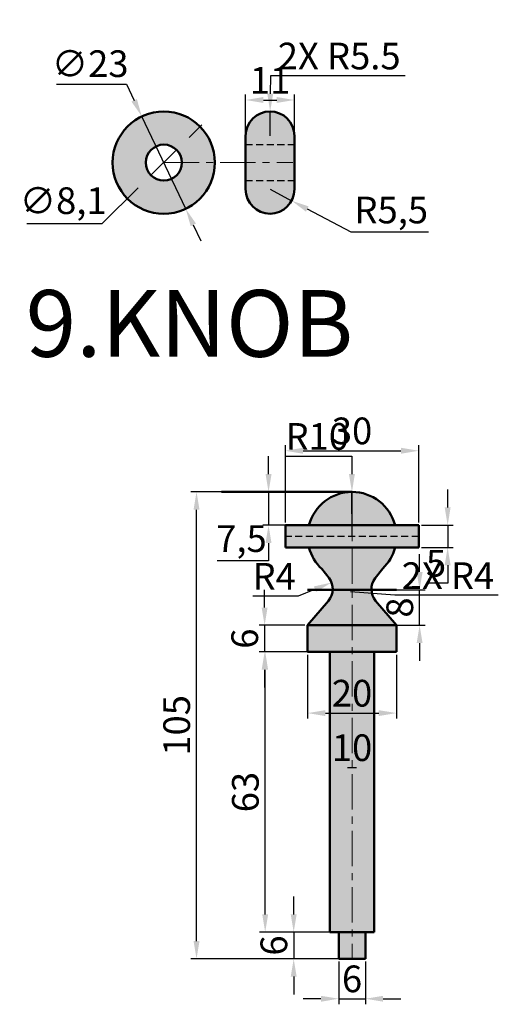
# Model space of a CAD drawing. Units: millimetres. Extents: x -14 to 1073, y -445 to 318.
# Tile 5 of 6: x 615 to 723, y -42 to 179. Entities that reach past the tile are written whole.
import ezdxf

# ---------------------------------------------------------------- set-up
doc = ezdxf.new("R2010")
doc.units = ezdxf.units.MM
doc.header["$LTSCALE"] = 0.5
doc.linetypes.add('CENTER', pattern=[50.8, 31.75, -6.35, 6.35, -6.35])
doc.linetypes.add('HIDDEN', pattern=[9.525, 6.35, -3.175])
for name, color, linetype, lineweight in [('M-CNTR', 1, 'CENTER', 18), ('M-DIMS', 2, 'Continuous', 25), ('M-HATC', 8, 'Continuous', 18), ('M-HIDN', 4, 'HIDDEN', 25), ('M-OUTL', 7, 'Continuous', 50), ('M-TEXT', 3, 'Continuous', 25)]:
    doc.layers.add(name, color=color, linetype=linetype, lineweight=lineweight)
doc.styles.get("Standard").update_dxf_attribs({"font": 'arial.ttf'})
doc.dimstyles.new('ISO-25', dxfattribs={"dimtxt": 6, "dimasz": 4, "dimexe": 1.25, "dimexo": 0.625, "dimtad": 1, "dimtoh": 1, "dimtxsty": 'Standard', "dimcen": 2.5, "dimadec": 0, "dimazin": 0, "dimtfac": 1, "dimtmove": 0, "dimatfit": 3, "dimfxl": 1, "dimarcsym": 0})

# ---------------------------------------------------------------- blocks, each defined once
blk = doc.blocks.new('*D47')
at = {"layer": 'Defpoints', "color": 0, "ltscale": 0.5, "transparency": 16777216}
for p in [(642.43, 157.61), (652.3, 136.84)]:
    blk.add_point(p, dxfattribs=at)
at = {"layer": 'M-DIMS', "color": 0, "lineweight": -2, "ltscale": 0.5, "transparency": 16777216}
for p, q in [((623.25, 164.84), (639, 164.84)), ((639, 164.84), (640.72, 161.22)), ((652.3, 136.84), (642.43, 157.61)), ((654.02, 133.22), (655.74, 129.61))]:
    blk.add_line(p, q, dxfattribs=at)
at = {"layer": 'M-DIMS', "color": 0, "ltscale": 0.5, "transparency": 16777216}
for points in [[(641.32, 161.51), (640.11, 160.94), (642.43, 157.61)], [(654.62, 133.51), (653.42, 132.94), (652.3, 136.84)]]:
    blk.add_solid(points, dxfattribs=at)
at = {"layer": 'M-DIMS', "color": 0, "ltscale": 0.5, "transparency": 16777216, "insert": (630.81, 168.69), "char_height": 6, "attachment_point": 5}
blk.add_mtext('∅23', dxfattribs=at)
blk = doc.blocks.new('*D48')
at = {"layer": 'Defpoints', "color": 0, "ltscale": 0.5, "transparency": 16777216}
for p in [(671.27, 141.22), (676.13, 138.66)]:
    blk.add_point(p, dxfattribs=at)
at = {"layer": 'M-DIMS', "color": 0, "lineweight": -2, "ltscale": 0.5, "transparency": 16777216}
for p, q in [((671.27, 141.22), (676.13, 138.66)), ((689.56, 131.57), (679.67, 136.79)), ((706.9, 131.57), (689.56, 131.57))]:
    blk.add_line(p, q, dxfattribs=at)
at = {"layer": 'M-DIMS', "color": 0, "ltscale": 0.5, "transparency": 16777216}
blk.add_solid([(679.98, 137.38), (679.36, 136.2), (676.13, 138.66)], dxfattribs=at)
at = {"layer": 'M-DIMS', "color": 0, "ltscale": 0.5, "transparency": 16777216, "insert": (698.54, 135.78), "char_height": 6, "attachment_point": 5}
blk.add_mtext('R5,5', dxfattribs=at)
blk = doc.blocks.new('*D49')
at = {"layer": 'Defpoints', "color": 0, "ltscale": 0.5, "transparency": 16777216}
for p in [(676.77, 161.3), (665.77, 147.22), (676.77, 147.22)]:
    blk.add_point(p, dxfattribs=at)
at = {"layer": 'M-DIMS', "color": 0, "lineweight": -2, "ltscale": 0.5, "transparency": 16777216}
for p, q in [((665.77, 147.85), (665.77, 162.55)), ((676.77, 147.85), (676.77, 162.55)), ((669.77, 161.3), (672.77, 161.3))]:
    blk.add_line(p, q, dxfattribs=at)
at = {"layer": 'M-DIMS', "color": 0, "ltscale": 0.5, "transparency": 16777216}
for points in [[(669.77, 161.97), (669.77, 160.64), (665.77, 161.3)], [(672.77, 161.97), (672.77, 160.64), (676.77, 161.3)]]:
    blk.add_solid(points, dxfattribs=at)
at = {"layer": 'M-DIMS', "color": 0, "ltscale": 0.5, "transparency": 16777216, "insert": (671.27, 164.94), "char_height": 6, "attachment_point": 5}
blk.add_mtext('11', dxfattribs=at)
blk = doc.blocks.new('*D50')
at = {"layer": 'Defpoints', "color": 0, "ltscale": 0.5, "transparency": 16777216}
for p in [(650.25, 150.07), (644.48, 144.38)]:
    blk.add_point(p, dxfattribs=at)
at = {"layer": 'M-DIMS', "color": 0, "lineweight": -2, "ltscale": 0.5, "transparency": 16777216}
for p, q in [((653.1, 152.87), (655.95, 155.68)), ((650.25, 150.07), (644.48, 144.38)), ((633.51, 133.56), (641.63, 141.57)), ((616.59, 133.56), (633.51, 133.56))]:
    blk.add_line(p, q, dxfattribs=at)
at = {"layer": 'M-DIMS', "color": 0, "ltscale": 0.5, "transparency": 16777216}
for points in [[(652.63, 153.35), (653.57, 152.4), (650.25, 150.07)], [(641.17, 142.05), (642.1, 141.1), (644.48, 144.38)]]:
    blk.add_solid(points, dxfattribs=at)
at = {"layer": 'M-DIMS', "color": 0, "ltscale": 0.5, "transparency": 16777216, "insert": (624.74, 137.89), "char_height": 6, "attachment_point": 5}
blk.add_mtext('∅8,1', dxfattribs=at)
blk = doc.blocks.new('*D51')
at = {"layer": 'Defpoints', "color": 0, "ltscale": 0.5, "transparency": 16777216}
for p in [(689.72, -25.82), (676.6, -31.82), (689.72, -31.82)]:
    blk.add_point(p, dxfattribs=at)
at = {"layer": 'M-DIMS', "color": 0, "lineweight": -2, "ltscale": 0.5, "transparency": 16777216}
for p, q in [((676.6, -21.82), (676.6, -17.82)), ((689.1, -25.82), (675.35, -25.82)), ((676.6, -25.82), (676.6, -31.82)), ((689.1, -31.82), (675.35, -31.82)), ((676.6, -35.82), (676.6, -39.82))]:
    blk.add_line(p, q, dxfattribs=at)
at = {"layer": 'M-DIMS', "color": 0, "ltscale": 0.5, "transparency": 16777216}
for points in [[(675.93, -21.82), (677.27, -21.82), (676.6, -25.82)], [(675.93, -35.82), (677.27, -35.82), (676.6, -31.82)]]:
    blk.add_solid(points, dxfattribs=at)
at = {"layer": 'M-DIMS', "color": 0, "ltscale": 0.5, "transparency": 16777216, "insert": (672.91, -28.82), "char_height": 6, "attachment_point": 5, "rotation": 90}
blk.add_mtext('6', dxfattribs=at)
blk = doc.blocks.new('*D52')
at = {"layer": 'Defpoints', "color": 0, "ltscale": 0.5, "transparency": 16777216}
for p in [(654.74, 73.18), (689.72, 73.18), (689.72, -31.82)]:
    blk.add_point(p, dxfattribs=at)
at = {"layer": 'M-DIMS', "color": 0, "lineweight": -2, "ltscale": 0.5, "transparency": 16777216}
for p, q in [((689.1, 73.18), (653.49, 73.18)), ((654.74, -27.82), (654.74, 69.18)), ((689.1, -31.82), (653.49, -31.82))]:
    blk.add_line(p, q, dxfattribs=at)
at = {"layer": 'M-DIMS', "color": 0, "ltscale": 0.5, "transparency": 16777216}
for points in [[(654.07, 69.18), (655.41, 69.18), (654.74, 73.18)], [(654.07, -27.82), (655.41, -27.82), (654.74, -31.82)]]:
    blk.add_solid(points, dxfattribs=at)
at = {"layer": 'M-DIMS', "color": 0, "ltscale": 0.5, "transparency": 16777216, "insert": (651.05, 20.68), "char_height": 6, "attachment_point": 5, "rotation": 90}
blk.add_mtext('105', dxfattribs=at)
blk = doc.blocks.new('*D53')
at = {"layer": 'Defpoints', "color": 0, "ltscale": 0.5, "transparency": 16777216}
for p in [(679.72, 43.18), (670.05, 37.18), (679.72, 37.18)]:
    blk.add_point(p, dxfattribs=at)
at = {"layer": 'M-DIMS', "color": 0, "lineweight": -2, "ltscale": 0.5, "transparency": 16777216}
for p, q in [((670.05, 47.18), (670.05, 51.18)), ((679.1, 43.18), (668.8, 43.18)), ((670.05, 43.18), (670.05, 37.18)), ((679.1, 37.18), (668.8, 37.18)), ((670.05, 33.18), (670.05, 29.18))]:
    blk.add_line(p, q, dxfattribs=at)
at = {"layer": 'M-DIMS', "color": 0, "ltscale": 0.5, "transparency": 16777216}
for points in [[(669.39, 47.18), (670.72, 47.18), (670.05, 43.18)], [(669.39, 33.18), (670.72, 33.18), (670.05, 37.18)]]:
    blk.add_solid(points, dxfattribs=at)
at = {"layer": 'M-DIMS', "color": 0, "ltscale": 0.5, "transparency": 16777216, "insert": (666.36, 40.18), "char_height": 6, "attachment_point": 5, "rotation": 90}
blk.add_mtext('6', dxfattribs=at)
blk = doc.blocks.new('*D54')
at = {"layer": 'Defpoints', "color": 0, "ltscale": 0.5, "transparency": 16777216}
for p in [(670.19, 37.18), (684.72, 37.18), (684.72, -25.82)]:
    blk.add_point(p, dxfattribs=at)
at = {"layer": 'M-DIMS', "color": 0, "lineweight": -2, "ltscale": 0.5, "transparency": 16777216}
for p, q in [((684.1, 37.18), (668.94, 37.18)), ((670.19, -21.82), (670.19, 33.18)), ((684.1, -25.82), (668.94, -25.82))]:
    blk.add_line(p, q, dxfattribs=at)
at = {"layer": 'M-DIMS', "color": 0, "ltscale": 0.5, "transparency": 16777216}
for points in [[(669.52, 33.18), (670.85, 33.18), (670.19, 37.18)], [(669.52, -21.82), (670.85, -21.82), (670.19, -25.82)]]:
    blk.add_solid(points, dxfattribs=at)
at = {"layer": 'M-DIMS', "color": 0, "ltscale": 0.5, "transparency": 16777216, "insert": (666.5, 5.68), "char_height": 6, "attachment_point": 5, "rotation": 90}
blk.add_mtext('63', dxfattribs=at)
blk = doc.blocks.new('*D55')
at = {"layer": 'Defpoints', "color": 0, "ltscale": 0.5, "transparency": 16777216}
for p in [(704.72, 65.68), (704.72, 60.68), (711.23, 60.68)]:
    blk.add_point(p, dxfattribs=at)
at = {"layer": 'M-DIMS', "color": 0, "lineweight": -2, "ltscale": 0.5, "transparency": 16777216}
for p, q in [((711.23, 69.68), (711.23, 73.68)), ((705.35, 65.68), (712.48, 65.68)), ((711.23, 65.68), (711.23, 60.68)), ((705.35, 60.68), (712.48, 60.68)), ((711.23, 56.68), (711.23, 52.68)), ((711.23, 52.68), (706.62, 52.68))]:
    blk.add_line(p, q, dxfattribs=at)
at = {"layer": 'M-DIMS', "color": 0, "ltscale": 0.5, "transparency": 16777216}
for points in [[(710.56, 69.68), (711.89, 69.68), (711.23, 65.68)], [(710.56, 56.68), (711.89, 56.68), (711.23, 60.68)]]:
    blk.add_solid(points, dxfattribs=at)
at = {"layer": 'M-DIMS', "color": 0, "ltscale": 0.5, "transparency": 16777216, "insert": (708.61, 56.36), "char_height": 6, "attachment_point": 5}
blk.add_mtext('5', dxfattribs=at)
blk = doc.blocks.new('*D56')
at = {"layer": 'Defpoints', "color": 0, "ltscale": 0.5, "transparency": 16777216}
for p in [(689.72, 73.18), (670.94, 65.68), (689.72, 65.68)]:
    blk.add_point(p, dxfattribs=at)
at = {"layer": 'M-DIMS', "color": 0, "lineweight": -2, "ltscale": 0.5, "transparency": 16777216}
for p, q in [((670.94, 77.18), (670.94, 81.18)), ((689.1, 73.18), (669.69, 73.18)), ((670.94, 73.18), (670.94, 65.68)), ((689.1, 65.68), (669.69, 65.68)), ((670.94, 61.68), (670.94, 57.68)), ((670.94, 57.68), (659.39, 57.68))]:
    blk.add_line(p, q, dxfattribs=at)
at = {"layer": 'M-DIMS', "color": 0, "ltscale": 0.5, "transparency": 16777216}
for points in [[(670.27, 77.18), (671.61, 77.18), (670.94, 73.18)], [(670.27, 61.68), (671.61, 61.68), (670.94, 65.68)]]:
    blk.add_solid(points, dxfattribs=at)
at = {"layer": 'M-DIMS', "color": 0, "ltscale": 0.5, "transparency": 16777216, "insert": (664.85, 61.9), "char_height": 6, "attachment_point": 5}
blk.add_mtext('7,5', dxfattribs=at)
blk = doc.blocks.new('*D57')
at = {"layer": 'Defpoints', "color": 0, "ltscale": 0.5, "transparency": 16777216}
for p in [(689.72, 51.18), (704.92, 51.18), (689.72, 43.18)]:
    blk.add_point(p, dxfattribs=at)
at = {"layer": 'M-DIMS', "color": 0, "lineweight": -2, "ltscale": 0.5, "transparency": 16777216}
for p, q in [((704.92, 55.18), (704.92, 59.18)), ((690.35, 51.18), (706.17, 51.18)), ((704.92, 43.18), (704.92, 51.18)), ((690.35, 43.18), (706.17, 43.18)), ((704.92, 39.18), (704.92, 35.18))]:
    blk.add_line(p, q, dxfattribs=at)
at = {"layer": 'M-DIMS', "color": 0, "ltscale": 0.5, "transparency": 16777216}
for points in [[(704.25, 55.18), (705.59, 55.18), (704.92, 51.18)], [(704.25, 39.18), (705.59, 39.18), (704.92, 43.18)]]:
    blk.add_solid(points, dxfattribs=at)
at = {"layer": 'M-DIMS', "color": 0, "ltscale": 0.5, "transparency": 16777216, "insert": (701.23, 47.18), "char_height": 6, "attachment_point": 5, "rotation": 90}
blk.add_mtext('8', dxfattribs=at)
blk = doc.blocks.new('*D58')
at = {"layer": 'Defpoints', "color": 0, "ltscale": 0.5, "transparency": 16777216}
for p in [(681.37, 51.3), (685.09, 52.79)]:
    blk.add_point(p, dxfattribs=at)
at = {"layer": 'M-DIMS', "color": 0, "lineweight": -2, "ltscale": 0.5, "transparency": 16777216}
for p, q in [((677.66, 49.81), (681.37, 51.3)), ((667.39, 49.81), (677.66, 49.81))]:
    blk.add_line(p, q, dxfattribs=at)
at = {"layer": 'M-DIMS', "color": 0, "ltscale": 0.5, "transparency": 16777216}
blk.add_solid([(681.13, 51.92), (681.62, 50.68), (685.09, 52.79)], dxfattribs=at)
at = {"layer": 'M-DIMS', "color": 0, "ltscale": 0.5, "transparency": 16777216, "insert": (672.21, 53.43), "char_height": 6, "attachment_point": 5}
blk.add_mtext('R4', dxfattribs=at)
blk = doc.blocks.new('*D59')
at = {"layer": 'Defpoints', "color": 0, "ltscale": 0.5, "transparency": 16777216}
for p in [(694.72, 11.19), (684.72, 9.89), (694.72, 9.89)]:
    blk.add_point(p, dxfattribs=at)
at = {"layer": 'M-DIMS', "color": 0, "lineweight": -2, "ltscale": 0.5, "transparency": 16777216}
for p, q in [((684.72, 10.52), (684.72, 12.44)), ((688.72, 11.19), (690.72, 11.19)), ((694.72, 10.52), (694.72, 12.44))]:
    blk.add_line(p, q, dxfattribs=at)
at = {"layer": 'M-DIMS', "color": 0, "ltscale": 0.5, "transparency": 16777216}
for points in [[(688.72, 11.86), (688.72, 10.53), (684.72, 11.19)], [(690.72, 11.86), (690.72, 10.53), (694.72, 11.19)]]:
    blk.add_solid(points, dxfattribs=at)
at = {"layer": 'M-DIMS', "color": 0, "ltscale": 0.5, "transparency": 16777216, "insert": (689.72, 14.88), "char_height": 6, "attachment_point": 5}
blk.add_mtext('10', dxfattribs=at)
blk = doc.blocks.new('*D60')
at = {"layer": 'Defpoints', "color": 0, "ltscale": 0.5, "transparency": 16777216}
for p in [(679.72, 37.18), (699.72, 37.18), (699.72, 23.44)]:
    blk.add_point(p, dxfattribs=at)
at = {"layer": 'M-DIMS', "color": 0, "lineweight": -2, "ltscale": 0.5, "transparency": 16777216}
for p, q in [((679.72, 36.55), (679.72, 22.19)), ((699.72, 36.55), (699.72, 22.19)), ((683.72, 23.44), (695.72, 23.44))]:
    blk.add_line(p, q, dxfattribs=at)
at = {"layer": 'M-DIMS', "color": 0, "ltscale": 0.5, "transparency": 16777216}
for points in [[(683.72, 24.1), (683.72, 22.77), (679.72, 23.44)], [(695.72, 24.1), (695.72, 22.77), (699.72, 23.44)]]:
    blk.add_solid(points, dxfattribs=at)
at = {"layer": 'M-DIMS', "color": 0, "ltscale": 0.5, "transparency": 16777216, "insert": (689.72, 27.13), "char_height": 6, "attachment_point": 5}
blk.add_mtext('20', dxfattribs=at)
blk = doc.blocks.new('*D61')
at = {"layer": 'Defpoints', "color": 0, "ltscale": 0.5, "transparency": 16777216}
for p in [(686.72, -31.82), (692.72, -31.82), (692.72, -40.79)]:
    blk.add_point(p, dxfattribs=at)
at = {"layer": 'M-DIMS', "color": 0, "lineweight": -2, "ltscale": 0.5, "transparency": 16777216}
for p, q in [((686.72, -32.45), (686.72, -42.04)), ((692.72, -32.45), (692.72, -42.04)), ((682.72, -40.79), (678.72, -40.79)), ((686.72, -40.79), (692.72, -40.79)), ((696.72, -40.79), (700.72, -40.79))]:
    blk.add_line(p, q, dxfattribs=at)
at = {"layer": 'M-DIMS', "color": 0, "ltscale": 0.5, "transparency": 16777216}
for points in [[(682.72, -40.13), (682.72, -41.46), (686.72, -40.79)], [(696.72, -40.13), (696.72, -41.46), (692.72, -40.79)]]:
    blk.add_solid(points, dxfattribs=at)
at = {"layer": 'M-DIMS', "color": 0, "ltscale": 0.5, "transparency": 16777216, "insert": (689.72, -37.1), "char_height": 6, "attachment_point": 5}
blk.add_mtext('6', dxfattribs=at)
blk = doc.blocks.new('*D80')
at = {"layer": 'Defpoints', "color": 0, "ltscale": 0.5, "transparency": 16777216}
for p in [(704.72, 82.43), (674.72, 65.68), (704.72, 65.68)]:
    blk.add_point(p, dxfattribs=at)
at = {"layer": 'M-DIMS', "color": 0, "lineweight": -2, "ltscale": 0.5, "transparency": 16777216}
for p, q in [((674.72, 66.3), (674.72, 83.68)), ((678.72, 82.43), (700.72, 82.43)), ((704.72, 66.3), (704.72, 83.68))]:
    blk.add_line(p, q, dxfattribs=at)
at = {"layer": 'M-DIMS', "color": 0, "ltscale": 0.5, "transparency": 16777216}
for points in [[(678.72, 83.1), (678.72, 81.76), (674.72, 82.43)], [(700.72, 83.1), (700.72, 81.76), (704.72, 82.43)]]:
    blk.add_solid(points, dxfattribs=at)
at = {"layer": 'M-DIMS', "color": 0, "ltscale": 0.5, "transparency": 16777216, "insert": (689.72, 86.12), "char_height": 6, "attachment_point": 5}
blk.add_mtext('30', dxfattribs=at)
blk = doc.blocks.new('*D85')
at = {"layer": 'Defpoints', "color": 0, "ltscale": 0.5, "transparency": 16777216}
for p in [(671.3, 158.72), (671.27, 153.22)]:
    blk.add_point(p, dxfattribs=at)
at = {"layer": 'M-DIMS', "color": 0, "lineweight": -2, "ltscale": 0.5, "transparency": 16777216}
for p, q in [((671.35, 166.72), (671.33, 162.72)), ((701.68, 166.72), (671.35, 166.72)), ((671.27, 153.22), (671.3, 158.72))]:
    blk.add_line(p, q, dxfattribs=at)
at = {"layer": 'M-DIMS', "color": 0, "ltscale": 0.5, "transparency": 16777216}
blk.add_solid([(670.66, 162.73), (671.99, 162.72), (671.3, 158.72)], dxfattribs=at)
at = {"layer": 'M-DIMS', "color": 0, "ltscale": 0.5, "transparency": 16777216, "insert": (686.83, 170.41), "char_height": 6, "attachment_point": 5}
blk.add_mtext('2X R5.5', dxfattribs=at)
blk = doc.blocks.new('*D94')
at = {"layer": 'Defpoints', "color": 0, "ltscale": 0.5, "transparency": 16777216}
for p in [(689.7, 73.18), (689.72, 63.18)]:
    blk.add_point(p, dxfattribs=at)
at = {"layer": 'M-DIMS', "color": 0, "lineweight": -2, "ltscale": 0.5, "transparency": 16777216}
for p, q in [((674.74, 81.18), (689.68, 81.18)), ((689.68, 81.18), (689.69, 77.18)), ((689.72, 63.18), (689.7, 73.18))]:
    blk.add_line(p, q, dxfattribs=at)
at = {"layer": 'M-DIMS', "color": 0, "ltscale": 0.5, "transparency": 16777216}
blk.add_solid([(690.36, 77.18), (689.03, 77.18), (689.7, 73.18)], dxfattribs=at)
at = {"layer": 'M-DIMS', "color": 0, "ltscale": 0.5, "transparency": 16777216, "insert": (681.9, 84.87), "char_height": 6, "attachment_point": 5}
blk.add_mtext('R10', dxfattribs=at)
blk = doc.blocks.new('*D95')
at = {"layer": 'Defpoints', "color": 0, "ltscale": 0.5, "transparency": 16777216}
for p in [(681.37, 51.3), (685.36, 51)]:
    blk.add_point(p, dxfattribs=at)
at = {"layer": 'M-DIMS', "color": 0, "lineweight": -2, "ltscale": 0.5, "transparency": 16777216}
for p, q in [((681.37, 51.3), (685.36, 51)), ((699.35, 49.92), (689.35, 50.69)), ((722.62, 49.92), (699.35, 49.92))]:
    blk.add_line(p, q, dxfattribs=at)
at = {"layer": 'M-DIMS', "color": 0, "ltscale": 0.5, "transparency": 16777216}
blk.add_solid([(689.4, 51.35), (689.3, 50.03), (685.36, 51)], dxfattribs=at)
at = {"layer": 'M-DIMS', "color": 0, "ltscale": 0.5, "transparency": 16777216, "insert": (711.3, 53.56), "char_height": 6, "attachment_point": 5}
blk.add_mtext('2X R4', dxfattribs=at)

msp = doc.modelspace()

# ---------------------------------------------------------------- hatches: boundary and pattern name
at = {"layer": 'M-HATC', "ltscale": 0.5}
h = msp.add_hatch(color=256, dxfattribs=at)
h.set_gradient(color1=(128, 128, 128), color2=(192, 192, 192), tint=1, name='INVCYLINDER')
h.paths.add_polyline_path([(635.8678, 147.2237, 1), (658.8678, 147.2237), (651.4178, 147.2237, -1), (643.3178, 147.2237, -1), (651.4178, 147.2237), (658.8678, 147.2237, 1)])
h.paths.add_polyline_path([(676.7698, 141.2237), (676.7698, 143.1737), (665.7698, 143.1737), (665.7698, 141.2237, 0.41421356), (671.2698, 135.7237, 0.41421356)])
h.paths.add_polyline_path([(676.7698, 153.2237, 0.41421356), (671.2698, 158.7237, 0.41421356), (665.7698, 153.2237), (665.7698, 151.2737), (676.7698, 151.2737)])
h.paths.add_polyline_path([(676.7698, 151.2737), (665.7698, 151.2737), (665.7698, 143.1737), (676.7698, 143.1737)])
h = msp.add_hatch(color=256, dxfattribs=at)
h.set_gradient(color1=(128, 128, 128), color2=(128, 128, 128), tint=1, name='INVCYLINDER')
h.paths.add_polyline_path([(689.7207, 73.1794, 0.34199871), (680.0382, 65.6794), (689.7207, 65.6794)])
h.paths.add_polyline_path([(689.7207, 73.1794), (689.7207, 65.6794), (699.4032, 65.6794, 0.34199871)])
h.paths.add_polyline_path([(689.7207, 60.6794), (680.0382, 60.6794, 0.14353764), (682.92, 55.8479), (684.5422, 53.7445, -0.17360102), (685.373, 51.1794), (689.7207, 51.1794)])
h.paths.add_polyline_path([(699.4032, 60.6794), (689.7207, 60.6794), (689.7207, 51.1794), (694.0762, 51.1794, -0.17395612), (694.9164, 53.7469), (696.6256, 55.9459, 0.1398892)])
h.paths.add_polyline_path([(689.7207, 63.1794), (674.7207, 63.1794), (674.7207, 60.6794), (689.7207, 60.6794)])
h.paths.add_polyline_path([(689.7207, 65.6794), (680.0382, 65.6794), (674.7207, 65.6794), (674.7207, 63.1794), (689.7207, 63.1794)])
h.paths.add_polyline_path([(704.7207, 65.6794), (689.7207, 65.6794), (689.7207, 63.1794), (704.7207, 63.1794)])
h.paths.add_polyline_path([(704.7207, 63.1794), (689.7207, 63.1794), (689.7207, 60.6794), (699.4032, 60.6794), (704.7207, 60.6794)])
h.paths.add_polyline_path([(695.0268, 48.7016, -0.17070158), (694.0762, 51.1794), (689.7207, 51.1794), (689.7207, 43.1794), (699.7207, 43.1794)])
h.paths.add_polyline_path([(689.7207, 51.1794), (685.373, 51.1794, -0.17009221), (684.4226, 48.711), (679.7207, 43.1794), (689.7207, 43.1794)])
h.paths.add_polyline_path([(689.7207, 43.1794), (679.7207, 43.1794), (679.7207, 37.1794), (689.7207, 37.1794)])
h.paths.add_polyline_path([(699.7207, 43.1794), (689.7207, 43.1794), (689.7207, 37.1794), (699.7207, 37.1794)])
h.paths.add_polyline_path([(689.7207, 37.1794), (684.7207, 37.1794), (684.7207, -25.8206), (689.7207, -25.8206)])
h.paths.add_polyline_path([(694.7207, 37.1794), (689.7207, 37.1794), (689.7207, -25.8206), (694.7207, -25.8206)])
h.paths.add_polyline_path([(689.7207, -25.8206), (686.7207, -25.8206), (686.7207, -31.8206), (689.7207, -31.8206)])
h.paths.add_polyline_path([(692.7207, -25.8206), (689.7207, -25.8206), (689.7207, -31.8206), (692.7207, -31.8206)])

# ---------------------------------------------------------------- linework, layer by layer
at = {"layer": 'M-CNTR', "ltscale": 0.5}
for p, q in [((647.3678, 147.2237), (676.4054, 147.2237)), ((689.7207, 73.1794), (689.7207, -31.8206))]:
    msp.add_line(p, q, dxfattribs=at)
at = {"layer": 'M-HIDN', "ltscale": 0.5}
for p, q in [((665.7698, 151.2737), (676.7698, 151.2737)), ((665.7698, 143.1737), (676.7698, 143.1737)), ((704.7207, 63.1794), (674.7207, 63.1794))]:
    msp.add_line(p, q, dxfattribs=at)
at = {"layer": 'M-OUTL', "ltscale": 0.5}
for p, q in [((671.2698, 158.7237), (671.2698, 158.7237)), ((665.7698, 153.2237), (665.7698, 141.2237)), ((676.7698, 141.2237), (676.7698, 153.2237)), ((671.2698, 135.7237), (671.2698, 135.7237)), ((660.3561, 73.1794), (689.7207, 73.1794)), ((674.7207, 65.6794), (704.7207, 65.6794)), ((674.7207, 60.6794), (674.7207, 65.6794)), ((689.7207, 65.6794), (704.7207, 65.6794)), ((704.7207, 65.6794), (704.7207, 60.6794)), ((704.7207, 60.6794), (674.7207, 60.6794)), ((684.5422, 53.7445), (682.92, 55.8479)), ((694.9164, 53.7469), (696.6256, 55.9459)), ((679.7207, 51.1794), (699.7207, 51.1794)), ((679.7207, 43.1794), (684.4226, 48.711)), ((699.7207, 43.1794), (695.0268, 48.7016)), ((679.7207, 43.1794), (699.7207, 43.1794)), ((679.7207, 37.1794), (679.7207, 43.1794)), ((699.7207, 43.1794), (699.7207, 37.1794)), ((699.7207, 37.1794), (679.7207, 37.1794)), ((684.7207, -25.8206), (684.7207, 37.1794)), ((694.7207, -25.8206), (694.7207, 37.1794)), ((684.7207, -25.8206), (694.7207, -25.8206)), ((686.7207, -31.8206), (686.7207, -25.8206)), ((692.7207, -31.8206), (692.7207, -25.8206)), ((686.7207, -31.8206), (692.7207, -31.8206))]:
    msp.add_line(p, q, dxfattribs=at)
for radius in [11.5, 4.05]:
    msp.add_circle((647.3678, 147.2237), radius, dxfattribs=at)
for centre, radius, start, end in [((671.2698, 153.2237), 5.5, 90, 180), ((671.2698, 153.2237), 5.5, 0, 90), ((671.2698, 141.2237), 5.5, 180, 270), ((671.2698, 141.2237), 5.5, 270, 0), ((689.7207, 63.1794), 10, 14.477512, 165.522488), ((689.7207, 63.1794), 10, 194.477512, 227.150746), ((689.7207, 63.1794), 10, 313.668952, 345.522488), ((681.3749, 51.3016), 4, 319.635463, 37.641997), ((698.0746, 51.2922), 4, 142.143289, 220.364537)]:
    msp.add_arc(centre, radius, start, end, dxfattribs=at)

# ---------------------------------------------------------------- texts
at = {"layer": 'M-TEXT', "ltscale": 0.5, "insert": (602.7162, 118.5648), "char_height": 15, "attachment_point": 1}
msp.add_mtext_dynamic_manual_height_columns('\\pxqc;9.KNOB', width=100.886837, gutter_width=12.5, heights=[0], dxfattribs=at)

# ---------------------------------------------------------------- dimensions: what is measured, and where the dimension line sits
at = {"layer": 'M-DIMS', "ltscale": 0.5}
for center, mpoint, override, picture, middle in [((671.2698, 153.2237), (671.3032, 158.7236), {"dimdec": 1, "dimlfac": 1, "dimrnd": 0, "dimzin": 0, "dimdsep": 46, "dimlunit": 2}, '*D85', (686.8294, 170.4119)), ((681.3749, 51.3016), (685.3632, 50.9957), {"dimdec": 0, "dimlfac": 1, "dimrnd": 0, "dimzin": 0, "dimdsep": 46, "dimlunit": 2}, '*D95', (711.2984, 53.5622))]:
    dim = msp.add_radius_dim(center=center, mpoint=mpoint, text='2X <>', dimstyle='ISO-25', override=override, dxfattribs=at)
    dim.commit()
    dim.dimension.update_dxf_attribs({"geometry": picture, "text_midpoint": middle})
for p1, p2, picture, middle in [((652.3024, 136.8362), (642.4332, 157.6111), '*D47', (630.814, 168.6935)), ((650.2522, 150.0667), (644.4834, 144.3806), '*D50', (624.7383, 137.8935))]:
    dim = msp.add_diameter_dim_2p(p1=p1, p2=p2, dimstyle='ISO-25', override={"dimclrd": 0, "dimclre": 0, "dimclrt": 0}, dxfattribs=at)
    dim.commit()
    dim.dimension.update_dxf_attribs({"geometry": picture, "text_midpoint": middle})
for base, p1, p2, override, picture, middle in [((676.7698, 161.3022), (665.7698, 147.2237), (676.7698, 147.2237), {"dimclrd": 0, "dimclre": 0, "dimclrt": 0}, '*D49', (671.2698, 164.9394)), ((704.7207, 82.4294), (674.7207, 65.6794), (704.7207, 65.6794), {"dimdec": 0, "dimlfac": 1, "dimrnd": 0, "dimzin": 0, "dimdsep": 46, "dimlunit": 2}, '*D80', (689.7207, 86.1198)), ((699.7207, 23.4374), (679.7207, 37.1794), (699.7207, 37.1794), {"dimclrd": 0, "dimclre": 0, "dimclrt": 0}, '*D60', (689.7207, 27.1258)), ((694.7207, 11.1947), (684.7207, 9.8922), (694.7207, 9.8922), {"dimclrd": 0, "dimclre": 0, "dimclrt": 0}, '*D59', (689.7207, 14.8831))]:
    dim = msp.add_linear_dim(base=base, p1=p1, p2=p2, dimstyle='ISO-25', override=override, dxfattribs=at)
    dim.commit()
    dim.dimension.update_dxf_attribs({"geometry": picture, "text_midpoint": middle})
for center, mpoint, override, picture, middle in [((671.2698, 141.2237), (676.1336, 138.656), {"dimclrd": 0, "dimclre": 0, "dimclrt": 0}, '*D48', (698.5444, 135.7846)), ((689.7207, 63.1794), (689.7, 73.1793), {"dimdec": 0, "dimlfac": 1, "dimrnd": 0, "dimzin": 0, "dimdsep": 46, "dimlunit": 2}, '*D94', (681.9003, 84.8678))]:
    dim = msp.add_radius_dim(center=center, mpoint=mpoint, dimstyle='ISO-25', override=override, dxfattribs=at)
    dim.commit()
    dim.dimension.update_dxf_attribs({"geometry": picture, "text_midpoint": middle})
for base, p1, p2, picture, middle in [((670.9385, 65.6794), (689.7207, 73.1794), (689.7207, 65.6794), '*D56', (664.8538, 61.8978)), ((654.7415, 73.1794), (689.7207, -31.8206), (689.7207, 73.1794), '*D52', (651.0531, 20.6794)), ((711.2268, 60.6794), (704.7207, 65.6794), (704.7207, 60.6794), '*D55', (708.6127, 56.3555)), ((704.921, 51.1794), (689.7207, 43.1794), (689.7207, 51.1794), '*D57', (701.2325, 47.1794)), ((670.0517, 37.1794), (679.7207, 43.1794), (679.7207, 37.1794), '*D53', (666.3632, 40.1794)), ((670.1869, 37.1794), (684.7207, -25.8206), (684.7207, 37.1794), '*D54', (666.4964, 5.6794)), ((676.6006, -31.8206), (689.7207, -25.8206), (689.7207, -31.8206), '*D51', (672.9122, -28.8206))]:
    dim = msp.add_linear_dim(base=base, p1=p1, p2=p2, angle=90, dimstyle='ISO-25', override={"dimclrd": 0, "dimclre": 0, "dimclrt": 0}, dxfattribs=at)
    dim.commit()
    dim.dimension.update_dxf_attribs({"geometry": picture, "text_midpoint": middle})
dim = msp.add_radius_dim(center=(681.3749, 51.3016), mpoint=(685.0857, 52.7948), dimstyle='ISO-25', override={"dimclrd": 0, "dimclre": 0, "dimclrt": 0}, dxfattribs=at)
dim.commit()
dim.dimension.update_dxf_attribs({"geometry": '*D58', "text_midpoint": (672.2136, 49.8085), "dimtype": 164})
dim = msp.add_linear_dim(base=(692.7207, -40.793), p1=(686.7207, -31.8206), p2=(692.7207, -31.8206), dimstyle='ISO-25', override={"dimclrd": 0, "dimclre": 0, "dimclrt": 0}, dxfattribs=at)
dim.commit()
dim.dimension.update_dxf_attribs({"geometry": '*D61', "text_midpoint": (689.7207, -40.793), "dimtype": 160})

doc.saveas('drawing.dxf')
